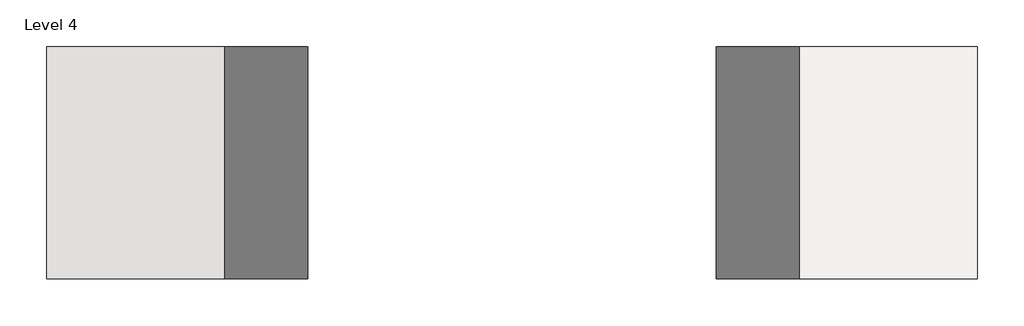
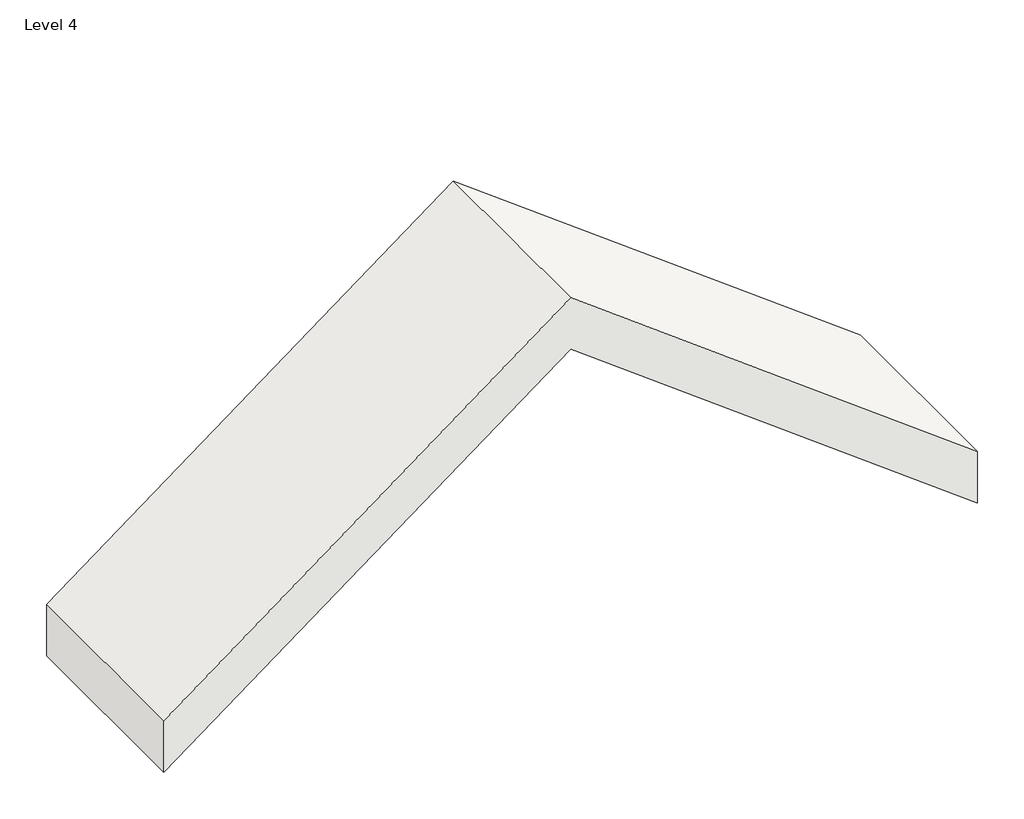
# One storey: 1 roof.
"""IFC4 building model written with IfcOpenShell, lengths in millimetres."""

from ifc_helpers import new_model, si_unit, frame, origin, place, context, project, spatial, polyline, outline, extrude, element, save

model = new_model("IFC4")

# Units and contexts
model_context = context("Model", 3, world=origin())
ifc_project = project(units=[si_unit("LENGTHUNIT", "METRE", prefix="MILLI")], contexts=[model_context])

# Site, building, storey
site = spatial("IfcSite", under=ifc_project)
building = spatial("IfcBuilding", under=site)
storey = spatial("IfcBuildingStorey", under=building, Name="Level 4", Elevation=9144.0)

# Roof
placement = place(None, origin())
element("IfcRoof", 1, ObjectType="Generic - 12\"", at=placement, inside=storey, context=model_context, shape_type="SweptSolid", body=[
    extrude(outline(polyline([(9525.0, -6863.5486248), (11661.6215913, -9712.3774133), (9525.0, -12561.2062017), (9144.0, -12561.2062017), (11280.6215913, -9712.3774133), (9144.0, -6863.5486248), (9525.0, -6863.5486248)])), frame((0.0, -13419.0040375, 0.0), z_axis=(0.0, 1.0, 0.0), x_axis=(0.0, 0.0, 1.0)), (0.0, 0.0, 1.0), 1422.4),
])

save(model, "model.ifc")

# Revit data of these elements
# Type "Generic - 12\""
#   Assembly Code = "B1020"
#   Layers, outside or top first: 1' - 0" no material (function 1)
# Element 1 (IfcRoof, "Generic - 12\"")
#   built-in parameter 1001705 = 38.2599 (stored number, unit not read)
#   built-in parameter 1001710 = 33615
#   Phase Created = New Construction
#   Materials on its faces: "Default Roof"
# Materials
#   "Default Roof": colour RGB 88 101 114, transparency 0, Cost = 0
